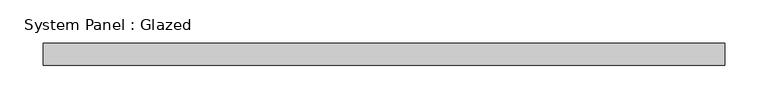
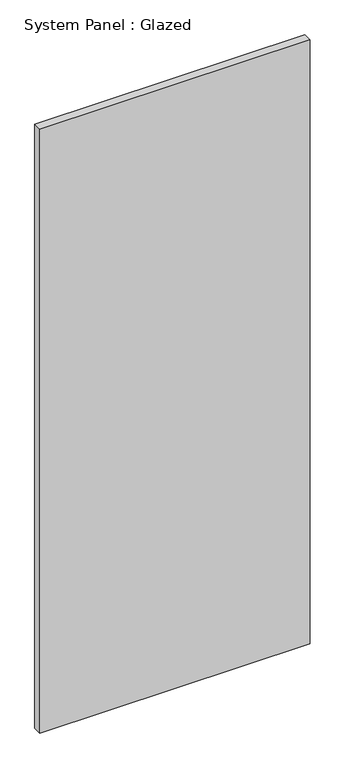
"""IFC4 building model written with IfcOpenShell, lengths in millimetres: plate geometry, System Panel : Glazed."""

from ifc_helpers import new_model, si_unit, origin, origin_with_axes, place, context, project, spatial, polyline, outline, extrude, source, transform, mapped, element, save


def system_panel_glazed_841e5d8e(model_context):
    return source(origin(), model_context, "Body", "SweptSolid", [
        extrude(outline(polyline([(393.7, 19.05), (-393.7, 19.05), (-393.7, 44.45), (393.7, 44.45), (393.7, 19.05)])), origin_with_axes(), (0.0, 0.0, 1.0), 1859.5412729),
    ])


if __name__ == "__main__":
    model = new_model("IFC4")
    model_context = context("Model", 3, world=origin())
    ifc_project = project(units=[si_unit("LENGTHUNIT", "METRE", prefix="MILLI")], contexts=[model_context])
    site = spatial("IfcSite", under=ifc_project)
    building = spatial("IfcBuilding", under=site)
    placement = place(None, origin())
    system_panel_glazed_shape = system_panel_glazed_841e5d8e(model_context)
    element("IfcPlate", 1, ObjectType="System Panel : Glazed", at=placement, inside=building, context=model_context, shape_type="MappedRepresentation", body=[
        mapped(system_panel_glazed_shape, transform((0.0, 0.0, 0.0), x_axis=(1.0, 0.0, 0.0), y_axis=(0.0, 1.0, 0.0), z_axis=(0.0, 0.0, 1.0))),
    ])
    save(model, "model.ifc")

# Revit data of these elements
# Type "System Panel : Glazed"
#   Construction Type Id = "GSP4R"
#   Analytic Construction = "1/8 in Pilkington single glazing"
#   Visual Light Transmittance = 0.9
#   Solar Heat Gain Coefficient = 0.86
#   Heat Transfer Coefficient (U) = 1.18115 BTU/(h·ft²·°F)
#   Define Thermal Properties by = 1
# Element 1 (IfcPlate, "System Panel : Glazed")
#   Materials on its faces: "Glass"
# Materials
#   "Glass": class "Glass", colour RGB 0 128 192, transparency 0.75, Description = "Soda Lime Glass", Cost = 0
